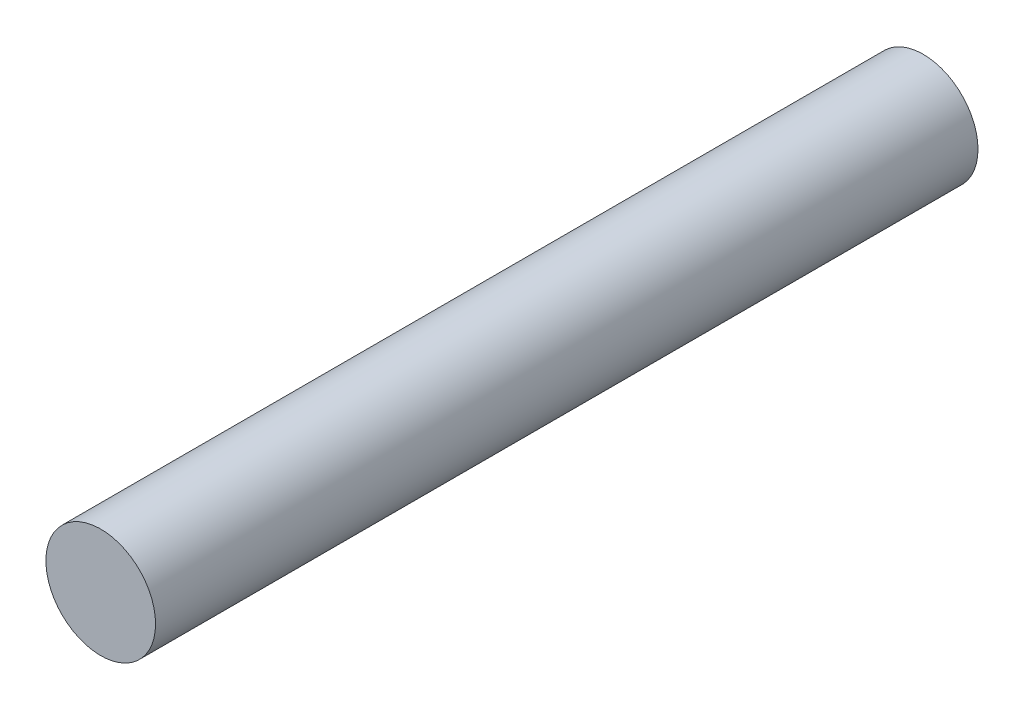
SolidWorks part; units mm, degrees
material "Plain Carbon Steel"
ref_plane "Front Plane" through (0, 0, 0) normal (0, 0, 1) x (1, 0, 0)
ref_plane "Top Plane" through (0, 0, 0) normal (0, 1, 0) x (1, 0, 0)
ref_plane "Right Plane" through (0, 0, 0) normal (1, 0, 0) x (0, 0, -1)
sketch "Pin Profile Ø4" plane through (0, 0, 0) normal (0, 0, 1) x (1, 0, 0)
  circle A0 centre (0, 0) radius 2
  dimension "D1" = 4
extrude "Pin Body Ø4x30" add sketch "Pin Profile Ø4" along normal blind 30
